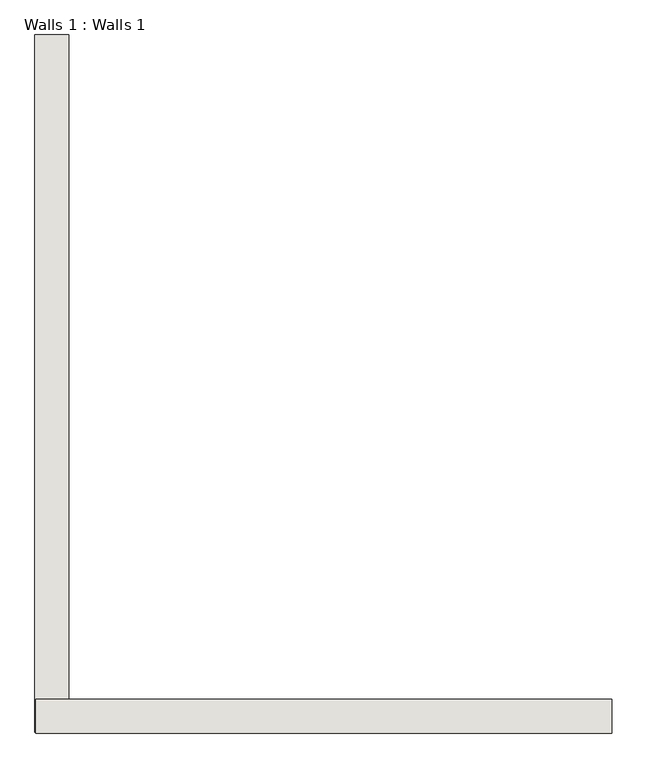
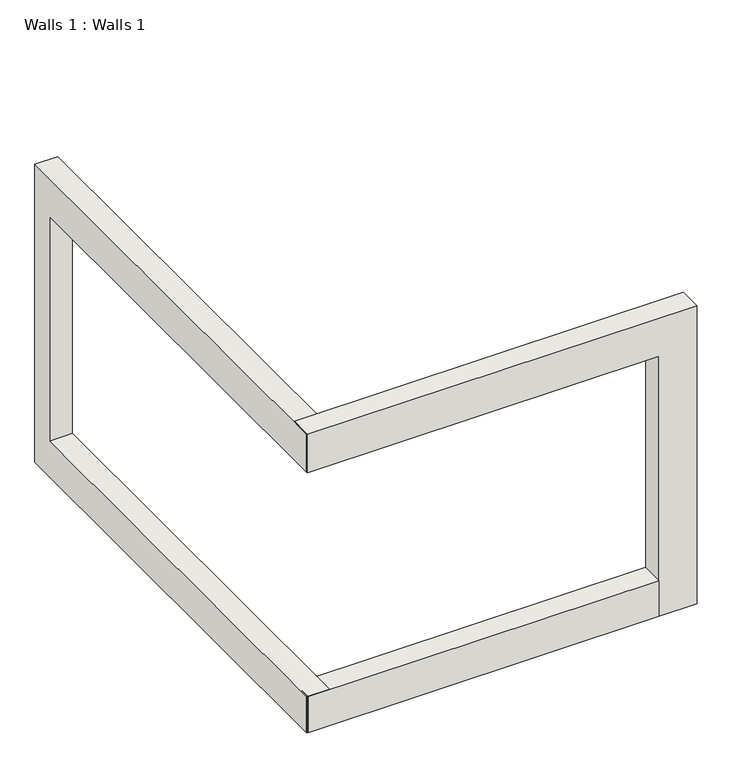
"""IFC4 building model written with IfcOpenShell, lengths in millimetres: wall geometry, Walls 1 : Walls 1."""

from ifc_helpers import new_model, si_unit, frame, origin, place, context, project, spatial, polyline, outline, extrude, source, transform, mapped, element, save


def walls_1_walls_1_33573b5d(model_context):
    return source(origin(), model_context, "Body", "SweptSolid", [
        extrude(outline(polyline([(5180.9930334, 4162.1385948), (5180.9930334, 7315.2), (-743.824816, 7315.2), (-743.824816, 7850.5521648), (5517.1742715, 7850.5521648), (5517.1742715, 3657.6), (-746.6059637, 3657.6), (-746.6059637, 4162.1385948), (5180.9930334, 4162.1385948)])), frame((-12861.2681702, 0.0, 0.0), z_axis=(1.0, 0.0, 0.0), x_axis=(0.0, 1.0, 0.0)), (0.0, 0.0, 1.0), 304.8),
        extrude(outline(polyline([(-8180.9078787, -754.1387835), (-12851.6122605, -754.1387835), (-12851.6122605, -449.3387835), (-8180.9078787, -449.3387835), (-8180.9078787, -754.1387835)])), frame((0.0, 0.0, 3657.6), z_axis=(0.0, 0.0, 1.0), x_axis=(1.0, 0.0, 0.0)), (0.0, 0.0, 1.0), 504.5385948),
        extrude(outline(polyline([(7851.9581577, -7679.6681702), (7851.9581577, -12852.7702358), (7315.2, -12852.7702358), (7315.2, -8180.9078787), (3657.6, -8180.9078787), (3657.6, -7679.6681702), (7851.9581577, -7679.6681702)])), frame((0.0, -754.1387835, 0.0), z_axis=(0.0, 1.0, 0.0), x_axis=(0.0, 0.0, 1.0)), (0.0, 0.0, 1.0), 304.8),
    ])


if __name__ == "__main__":
    model = new_model("IFC4")
    model_context = context("Model", 3, world=origin())
    ifc_project = project(units=[si_unit("LENGTHUNIT", "METRE", prefix="MILLI")], contexts=[model_context])
    site = spatial("IfcSite", under=ifc_project)
    building = spatial("IfcBuilding", under=site)
    placement = place(None, origin())
    walls_1_walls_1_shape = walls_1_walls_1_33573b5d(model_context)
    element("IfcWall", 1, ObjectType="Walls 1 : Walls 1", at=placement, inside=building, context=model_context, shape_type="MappedRepresentation", body=[
        mapped(walls_1_walls_1_shape, transform((0.0, 0.0, 0.0), x_axis=(1.0, 0.0, 0.0), y_axis=(0.0, 1.0, 0.0), z_axis=(0.0, 0.0, 1.0))),
    ])
    save(model, "model.ifc")

# Revit data of these elements
# Element 1 (IfcWall, "Walls 1 : Walls 1")
#   Materials on its faces: "Default Wall"
# Materials
#   "Default Wall": colour RGB 128 128 128, transparency 0
